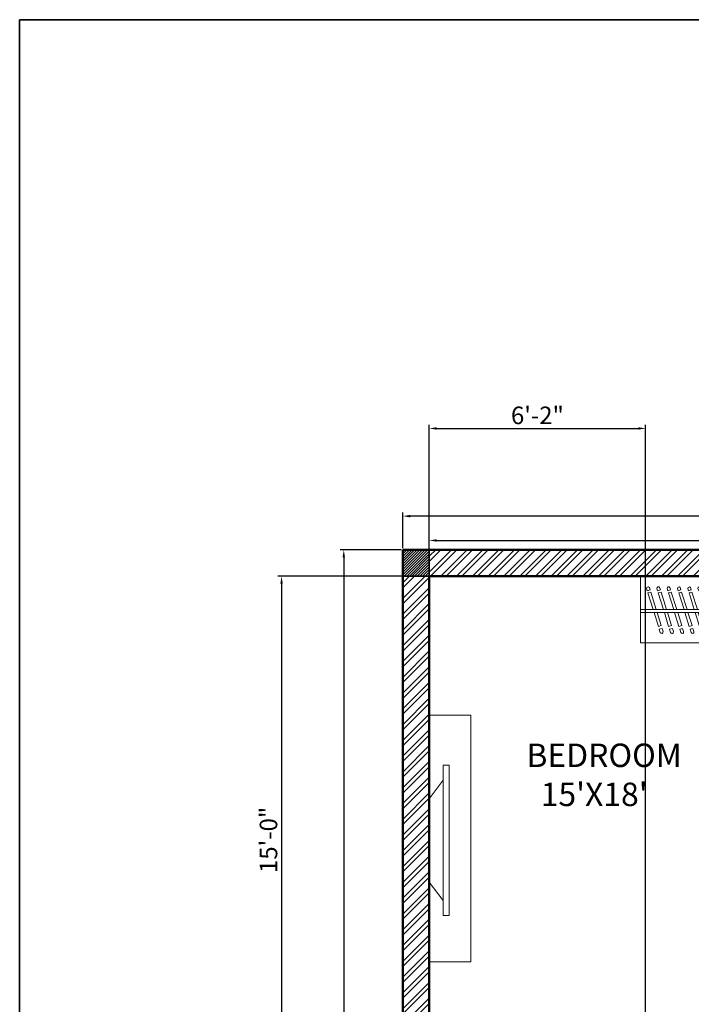
# Model space of a CAD drawing. Units: millimetres. Extents: x 20768 to 23556, y 50760 to 52704.
# Tile 21 of 36: x 20768 to 20998, y 52368 to 52704. Entities that reach past the tile are written whole.
import ezdxf

# ---------------------------------------------------------------- set-up
doc = ezdxf.new("R2010")
doc.units = ezdxf.units.MM
for name, color, linetype, lineweight in [('A-ANNO-DIMS', 2, 'Continuous', 18), ('A-ANNO-TTLB', 7, 'Continuous', 35), ('A-AREA-IDEN', 40, 'Continuous', 18), ('A-FURN', 8, 'Continuous', 18), ('A-WALL', 7, 'Continuous', 50), ('A-WALL-PATT', 8, 'Continuous', 13), ('S-ANNO-DIMS', 2, 'Continuous', 18), ('S-COLS', 20, 'Continuous', 35)]:
    doc.layers.add(name, color=color, linetype=linetype, lineweight=lineweight)
doc.styles.get("Standard").update_dxf_attribs({"font": 'arial.ttf'})
doc.dimstyles.new('ISO-25', dxfattribs={"dimtxt": 6, "dimasz": 2.5, "dimexe": 1.25, "dimexo": 0.625, "dimtad": 1, "dimdec": 0, "dimlunit": 3, "dimtxsty": 'Standard', "dimcen": 2.5, "dimadec": 0, "dimazin": 0, "dimtfac": 1, "dimtdec": 0, "dimtmove": 0, "dimatfit": 3, "dimfxl": 1, "dimarcsym": 0})
pattern_1 = [(45, (-81.1113, 0), (-2.69407684, 2.69407684), []), (45, (-79.3152, 0), (-2.69407684, 2.69407684), [])]

# ---------------------------------------------------------------- blocks, each defined once
blk = doc.blocks.new('wb')
for p, q in [((21205.25, 52502.52), (21061.44, 52502.52)), ((21205.25, 52501.52), (21061.44, 52501.52))]:
    blk.add_line(p, q)
blk.add_lwpolyline([(21205.25, 52513.9), (21061.44, 52513.9), (21061.44, 52491.15), (21205.25, 52491.15)], close=True)
for points in [[(21064.45, 52510.07, 0.695903), (21063.5, 52509.77), (21063.75, 52508.98), (21064.7, 52509.27)], [(21067.97, 52510.07, 0.695903), (21067.01, 52509.77), (21067.26, 52508.98), (21068.21, 52509.27)], [(21071.48, 52510.07, 0.695903), (21070.52, 52509.77), (21070.77, 52508.98), (21071.73, 52509.27)], [(21074.99, 52510.07, 0.695903), (21074.04, 52509.77), (21074.28, 52508.98), (21075.24, 52509.27)], [(21078.5, 52510.07, 0.695903), (21077.55, 52509.77), (21077.8, 52508.98), (21078.75, 52509.27)], [(21082.02, 52510.07, 0.695903), (21081.06, 52509.77), (21081.31, 52508.98), (21082.26, 52509.27)], [(21085.53, 52510.07, 0.695903), (21084.57, 52509.77), (21084.82, 52508.98), (21085.78, 52509.27)], [(21089.04, 52510.07, 0.695903), (21088.09, 52509.77), (21088.33, 52508.98), (21089.29, 52509.27)], [(21092.55, 52510.07, 0.695903), (21091.6, 52509.77), (21091.85, 52508.98), (21092.8, 52509.27)], [(21096.07, 52510.07, 0.695903), (21095.11, 52509.77), (21095.36, 52508.98), (21096.31, 52509.27)], [(21099.58, 52510.07, 0.695903), (21098.62, 52509.77), (21098.87, 52508.98), (21099.83, 52509.27)], [(21103.09, 52510.07, 0.695903), (21102.14, 52509.77), (21102.38, 52508.98), (21103.34, 52509.27)], [(21106.6, 52510.07, 0.695903), (21105.65, 52509.77), (21105.9, 52508.98), (21106.85, 52509.27)], [(21110.12, 52510.07, 0.695903), (21109.16, 52509.77), (21109.41, 52508.98), (21110.36, 52509.27)], [(21113.63, 52510.07, 0.695903), (21112.67, 52509.77), (21112.92, 52508.98), (21113.88, 52509.27)], [(21117.14, 52510.07, 0.695903), (21116.19, 52509.77), (21116.43, 52508.98), (21117.39, 52509.27)], [(21120.65, 52510.07, 0.695903), (21119.7, 52509.77), (21119.95, 52508.98), (21120.9, 52509.27)], [(21124.17, 52510.07, 0.695903), (21123.21, 52509.77), (21123.46, 52508.98), (21124.41, 52509.27)], [(21127.68, 52510.07, 0.695903), (21126.72, 52509.77), (21126.97, 52508.98), (21127.93, 52509.27)], [(21131.19, 52510.07, 0.695903), (21130.24, 52509.77), (21130.48, 52508.98), (21131.44, 52509.27)], [(21134.7, 52510.07, 0.695903), (21133.75, 52509.77), (21134, 52508.98), (21134.95, 52509.27)], [(21138.22, 52510.07, 0.695903), (21137.26, 52509.77), (21137.51, 52508.98), (21138.46, 52509.27)], [(21141.73, 52510.07, 0.695903), (21140.77, 52509.77), (21141.02, 52508.98), (21141.98, 52509.27)], [(21145.24, 52510.07, 0.695903), (21144.29, 52509.77), (21144.54, 52508.98), (21145.49, 52509.27)], [(21148.75, 52510.07, 0.695903), (21147.8, 52509.77), (21148.05, 52508.98), (21149, 52509.27)], [(21152.27, 52510.07, 0.695903), (21151.31, 52509.77), (21151.56, 52508.98), (21152.52, 52509.27)], [(21155.78, 52510.07, 0.695903), (21154.83, 52509.77), (21155.07, 52508.98), (21156.03, 52509.27)], [(21159.29, 52510.07, 0.695903), (21158.34, 52509.77), (21158.59, 52508.98), (21159.54, 52509.27)], [(21162.8, 52510.07, 0.695903), (21161.85, 52509.77), (21162.1, 52508.98), (21163.05, 52509.27)], [(21166.32, 52510.07, 0.695903), (21165.36, 52509.77), (21165.61, 52508.98), (21166.57, 52509.27)], [(21169.83, 52510.07, 0.695903), (21168.88, 52509.77), (21169.12, 52508.98), (21170.08, 52509.27)], [(21173.34, 52510.07, 0.695903), (21172.39, 52509.77), (21172.64, 52508.98), (21173.59, 52509.27)], [(21176.86, 52510.07, 0.695903), (21175.9, 52509.77), (21176.15, 52508.98), (21177.1, 52509.27)], [(21180.37, 52510.07, 0.695903), (21179.41, 52509.77), (21179.66, 52508.98), (21180.62, 52509.27)], [(21183.88, 52510.07, 0.695903), (21182.93, 52509.77), (21183.17, 52508.98), (21184.13, 52509.27)], [(21187.39, 52510.07, 0.695903), (21186.44, 52509.77), (21186.69, 52508.98), (21187.64, 52509.27)], [(21190.91, 52510.07, 0.695903), (21189.95, 52509.77), (21190.2, 52508.98), (21191.15, 52509.27)], [(21194.42, 52510.07, 0.695903), (21193.46, 52509.77), (21193.71, 52508.98), (21194.67, 52509.27)], [(21197.93, 52510.07, 0.695903), (21196.98, 52509.77), (21197.22, 52508.98), (21198.18, 52509.27)], [(21068.81, 52496.1), (21067.85, 52495.8), (21068.19, 52494.73, 1), (21069.14, 52495.03)], [(21072.32, 52496.1), (21071.37, 52495.8), (21071.7, 52494.73, 1), (21072.65, 52495.03)], [(21075.83, 52496.1), (21074.88, 52495.8), (21075.21, 52494.73, 1), (21076.17, 52495.03)], [(21079.35, 52496.1), (21078.39, 52495.8), (21078.73, 52494.73, 1), (21079.68, 52495.03)], [(21082.86, 52496.1), (21081.9, 52495.8), (21082.24, 52494.73, 1), (21083.19, 52495.03)], [(21086.37, 52496.1), (21085.42, 52495.8), (21085.75, 52494.73, 1), (21086.7, 52495.03)], [(21089.88, 52496.1), (21088.93, 52495.8), (21089.26, 52494.73, 1), (21090.22, 52495.03)], [(21093.4, 52496.1), (21092.44, 52495.8), (21092.78, 52494.73, 1), (21093.73, 52495.03)], [(21096.91, 52496.1), (21095.95, 52495.8), (21096.29, 52494.73, 1), (21097.24, 52495.03)], [(21100.42, 52496.1), (21099.47, 52495.8), (21099.8, 52494.73, 1), (21100.76, 52495.03)], [(21103.93, 52496.1), (21102.98, 52495.8), (21103.31, 52494.73, 1), (21104.27, 52495.03)], [(21107.45, 52496.1), (21106.49, 52495.8), (21106.83, 52494.73, 1), (21107.78, 52495.03)], [(21110.96, 52496.1), (21110, 52495.8), (21110.34, 52494.73, 1), (21111.29, 52495.03)], [(21114.47, 52496.1), (21113.52, 52495.8), (21113.85, 52494.73, 1), (21114.81, 52495.03)], [(21117.98, 52496.1), (21117.03, 52495.8), (21117.36, 52494.73, 1), (21118.32, 52495.03)], [(21121.5, 52496.1), (21120.54, 52495.8), (21120.88, 52494.73, 1), (21121.83, 52495.03)], [(21125.01, 52496.1), (21124.05, 52495.8), (21124.39, 52494.73, 1), (21125.34, 52495.03)], [(21128.52, 52496.1), (21127.57, 52495.8), (21127.9, 52494.73, 1), (21128.86, 52495.03)], [(21132.03, 52496.1), (21131.08, 52495.8), (21131.41, 52494.73, 1), (21132.37, 52495.03)], [(21135.55, 52496.1), (21134.59, 52495.8), (21134.93, 52494.73, 1), (21135.88, 52495.03)], [(21139.06, 52496.1), (21138.1, 52495.8), (21138.44, 52494.73, 1), (21139.39, 52495.03)], [(21142.57, 52496.1), (21141.62, 52495.8), (21141.95, 52494.73, 1), (21142.91, 52495.03)], [(21146.08, 52496.1), (21145.13, 52495.8), (21145.46, 52494.73, 1), (21146.42, 52495.03)], [(21149.6, 52496.1), (21148.64, 52495.8), (21148.98, 52494.73, 1), (21149.93, 52495.03)], [(21153.11, 52496.1), (21152.15, 52495.8), (21152.49, 52494.73, 1), (21153.44, 52495.03)], [(21156.62, 52496.1), (21155.67, 52495.8), (21156, 52494.73, 1), (21156.96, 52495.03)], [(21160.13, 52496.1), (21159.18, 52495.8), (21159.51, 52494.73, 1), (21160.47, 52495.03)], [(21163.65, 52496.1), (21162.69, 52495.8), (21163.03, 52494.73, 1), (21163.98, 52495.03)], [(21167.16, 52496.1), (21166.2, 52495.8), (21166.54, 52494.73, 1), (21167.49, 52495.03)], [(21170.67, 52496.1), (21169.72, 52495.8), (21170.05, 52494.73, 1), (21171.01, 52495.03)], [(21174.18, 52496.1), (21173.23, 52495.8), (21173.56, 52494.73, 1), (21174.52, 52495.03)], [(21177.7, 52496.1), (21176.74, 52495.8), (21177.08, 52494.73, 1), (21178.03, 52495.03)], [(21181.21, 52496.1), (21180.25, 52495.8), (21180.59, 52494.73, 1), (21181.54, 52495.03)], [(21184.72, 52496.1), (21183.77, 52495.8), (21184.1, 52494.73, 1), (21185.06, 52495.03)], [(21188.23, 52496.1), (21187.28, 52495.8), (21187.61, 52494.73, 1), (21188.57, 52495.03)], [(21191.75, 52496.1), (21190.79, 52495.8), (21191.13, 52494.73, 1), (21192.08, 52495.03)], [(21195.26, 52496.1), (21194.31, 52495.8), (21194.64, 52494.73, 1), (21195.59, 52495.03)], [(21198.77, 52496.1), (21197.82, 52495.8), (21198.15, 52494.73, 1), (21199.11, 52495.03)], [(21202.29, 52496.1), (21201.33, 52495.8), (21201.67, 52494.73, 1), (21202.62, 52495.03)]]:
    blk.add_lwpolyline(points, format="xyb", close=True)
for points in [[(21065.76, 52502.52), (21063.98, 52508.23), (21064.93, 52508.53), (21066.81, 52502.52)], [(21069.27, 52502.52), (21067.49, 52508.23), (21068.44, 52508.53), (21070.32, 52502.52)], [(21072.78, 52502.52), (21071, 52508.23), (21071.96, 52508.53), (21073.83, 52502.52)], [(21076.3, 52502.52), (21074.51, 52508.23), (21075.47, 52508.53), (21077.34, 52502.52)], [(21079.81, 52502.52), (21078.03, 52508.23), (21078.98, 52508.53), (21080.86, 52502.52)], [(21083.32, 52502.52), (21081.54, 52508.23), (21082.49, 52508.53), (21084.37, 52502.52)], [(21086.83, 52502.52), (21085.05, 52508.23), (21086.01, 52508.53), (21087.88, 52502.52)], [(21090.35, 52502.52), (21088.57, 52508.23), (21089.52, 52508.53), (21091.39, 52502.52)], [(21093.86, 52502.52), (21092.08, 52508.23), (21093.03, 52508.53), (21094.91, 52502.52)], [(21097.37, 52502.52), (21095.59, 52508.23), (21096.55, 52508.53), (21098.42, 52502.52)], [(21100.88, 52502.52), (21099.1, 52508.23), (21100.06, 52508.53), (21101.93, 52502.52)], [(21104.4, 52502.52), (21102.62, 52508.23), (21103.57, 52508.53), (21105.44, 52502.52)], [(21107.91, 52502.52), (21106.13, 52508.23), (21107.08, 52508.53), (21108.96, 52502.52)], [(21111.42, 52502.52), (21109.64, 52508.23), (21110.6, 52508.53), (21112.47, 52502.52)], [(21114.93, 52502.52), (21113.15, 52508.23), (21114.11, 52508.53), (21115.98, 52502.52)], [(21118.45, 52502.52), (21116.67, 52508.23), (21117.62, 52508.53), (21119.49, 52502.52)], [(21121.96, 52502.52), (21120.18, 52508.23), (21121.13, 52508.53), (21123.01, 52502.52)], [(21125.47, 52502.52), (21123.69, 52508.23), (21124.65, 52508.53), (21126.52, 52502.52)], [(21128.98, 52502.52), (21127.2, 52508.23), (21128.16, 52508.53), (21130.03, 52502.52)], [(21132.5, 52502.52), (21130.72, 52508.23), (21131.67, 52508.53), (21133.54, 52502.52)], [(21136.01, 52502.52), (21134.23, 52508.23), (21135.18, 52508.53), (21137.06, 52502.52)], [(21139.52, 52502.52), (21137.74, 52508.23), (21138.7, 52508.53), (21140.57, 52502.52)], [(21143.03, 52502.52), (21141.25, 52508.23), (21142.21, 52508.53), (21144.08, 52502.52)], [(21146.55, 52502.52), (21144.77, 52508.23), (21145.72, 52508.53), (21147.59, 52502.52)], [(21150.06, 52502.52), (21148.28, 52508.23), (21149.23, 52508.53), (21151.11, 52502.52)], [(21153.57, 52502.52), (21151.79, 52508.23), (21152.75, 52508.53), (21154.62, 52502.52)], [(21157.08, 52502.52), (21155.3, 52508.23), (21156.26, 52508.53), (21158.13, 52502.52)], [(21160.6, 52502.52), (21158.82, 52508.23), (21159.77, 52508.53), (21161.64, 52502.52)], [(21164.11, 52502.52), (21162.33, 52508.23), (21163.28, 52508.53), (21165.16, 52502.52)], [(21167.62, 52502.52), (21165.84, 52508.23), (21166.8, 52508.53), (21168.67, 52502.52)], [(21171.13, 52502.52), (21169.35, 52508.23), (21170.31, 52508.53), (21172.18, 52502.52)], [(21174.65, 52502.52), (21172.87, 52508.23), (21173.82, 52508.53), (21175.69, 52502.52)], [(21178.16, 52502.52), (21176.38, 52508.23), (21177.33, 52508.53), (21179.21, 52502.52)], [(21181.67, 52502.52), (21179.89, 52508.23), (21180.85, 52508.53), (21182.72, 52502.52)], [(21185.19, 52502.52), (21183.4, 52508.23), (21184.36, 52508.53), (21186.23, 52502.52)], [(21188.7, 52502.52), (21186.92, 52508.23), (21187.87, 52508.53), (21189.75, 52502.52)], [(21192.21, 52502.52), (21190.43, 52508.23), (21191.38, 52508.53), (21193.26, 52502.52)], [(21195.72, 52502.52), (21193.94, 52508.23), (21194.9, 52508.53), (21196.77, 52502.52)], [(21199.24, 52502.52), (21197.46, 52508.23), (21198.41, 52508.53), (21200.28, 52502.52)], [(21066.07, 52501.52), (21067.54, 52496.81), (21068.49, 52497.1), (21067.12, 52501.52)], [(21069.58, 52501.52), (21071.05, 52496.81), (21072.01, 52497.1), (21070.63, 52501.52)], [(21073.09, 52501.52), (21074.57, 52496.81), (21075.52, 52497.1), (21074.14, 52501.52)], [(21076.61, 52501.52), (21078.08, 52496.81), (21079.03, 52497.1), (21077.65, 52501.52)], [(21080.12, 52501.52), (21081.59, 52496.81), (21082.55, 52497.1), (21081.17, 52501.52)], [(21083.63, 52501.52), (21085.1, 52496.81), (21086.06, 52497.1), (21084.68, 52501.52)], [(21087.14, 52501.52), (21088.62, 52496.81), (21089.57, 52497.1), (21088.19, 52501.52)], [(21090.66, 52501.52), (21092.13, 52496.81), (21093.08, 52497.1), (21091.7, 52501.52)], [(21094.17, 52501.52), (21095.64, 52496.81), (21096.6, 52497.1), (21095.22, 52501.52)], [(21097.68, 52501.52), (21099.15, 52496.81), (21100.11, 52497.1), (21098.73, 52501.52)], [(21101.2, 52501.52), (21102.67, 52496.81), (21103.62, 52497.1), (21102.24, 52501.52)], [(21104.71, 52501.52), (21106.18, 52496.81), (21107.13, 52497.1), (21105.76, 52501.52)], [(21108.22, 52501.52), (21109.69, 52496.81), (21110.65, 52497.1), (21109.27, 52501.52)], [(21111.73, 52501.52), (21113.2, 52496.81), (21114.16, 52497.1), (21112.78, 52501.52)], [(21115.25, 52501.52), (21116.72, 52496.81), (21117.67, 52497.1), (21116.29, 52501.52)], [(21118.76, 52501.52), (21120.23, 52496.81), (21121.18, 52497.1), (21119.81, 52501.52)], [(21122.27, 52501.52), (21123.74, 52496.81), (21124.7, 52497.1), (21123.32, 52501.52)], [(21125.78, 52501.52), (21127.25, 52496.81), (21128.21, 52497.1), (21126.83, 52501.52)], [(21129.3, 52501.52), (21130.77, 52496.81), (21131.72, 52497.1), (21130.34, 52501.52)], [(21132.81, 52501.52), (21134.28, 52496.81), (21135.23, 52497.1), (21133.86, 52501.52)], [(21136.32, 52501.52), (21137.79, 52496.81), (21138.75, 52497.1), (21137.37, 52501.52)], [(21139.83, 52501.52), (21141.3, 52496.81), (21142.26, 52497.1), (21140.88, 52501.52)], [(21143.35, 52501.52), (21144.82, 52496.81), (21145.77, 52497.1), (21144.39, 52501.52)], [(21146.86, 52501.52), (21148.33, 52496.81), (21149.28, 52497.1), (21147.91, 52501.52)], [(21150.37, 52501.52), (21151.84, 52496.81), (21152.8, 52497.1), (21151.42, 52501.52)], [(21153.88, 52501.52), (21155.35, 52496.81), (21156.31, 52497.1), (21154.93, 52501.52)], [(21157.4, 52501.52), (21158.87, 52496.81), (21159.82, 52497.1), (21158.44, 52501.52)], [(21160.91, 52501.52), (21162.38, 52496.81), (21163.33, 52497.1), (21161.96, 52501.52)], [(21164.42, 52501.52), (21165.89, 52496.81), (21166.85, 52497.1), (21165.47, 52501.52)], [(21167.93, 52501.52), (21169.4, 52496.81), (21170.36, 52497.1), (21168.98, 52501.52)], [(21171.45, 52501.52), (21172.92, 52496.81), (21173.87, 52497.1), (21172.49, 52501.52)], [(21174.96, 52501.52), (21176.43, 52496.81), (21177.38, 52497.1), (21176.01, 52501.52)], [(21178.47, 52501.52), (21179.94, 52496.81), (21180.9, 52497.1), (21179.52, 52501.52)], [(21181.98, 52501.52), (21183.46, 52496.81), (21184.41, 52497.1), (21183.03, 52501.52)], [(21185.5, 52501.52), (21186.97, 52496.81), (21187.92, 52497.1), (21186.54, 52501.52)], [(21189.01, 52501.52), (21190.48, 52496.81), (21191.43, 52497.1), (21190.06, 52501.52)], [(21192.52, 52501.52), (21193.99, 52496.81), (21194.95, 52497.1), (21193.57, 52501.52)], [(21196.03, 52501.52), (21197.51, 52496.81), (21198.46, 52497.1), (21197.08, 52501.52)], [(21199.55, 52501.52), (21201.02, 52496.81), (21201.97, 52497.1), (21200.59, 52501.52)]]:
    blk.add_lwpolyline(points)
blk = doc.blocks.new('tv')
for p, q in [((20989.25, 52437.95), (20993.93, 52444.3)), ((20989.25, 52409.51), (20993.93, 52403.15))]:
    blk.add_line(p, q)
for points in [[(20989.25, 52466.51), (21003.46, 52466.51), (21003.46, 52382.21), (20989.25, 52382.21)], [(20993.93, 52449.42), (20996.05, 52449.42), (20996.05, 52398.03), (20993.93, 52398.03)]]:
    blk.add_lwpolyline(points, close=True)
blk = doc.blocks.new('*D108')
at = {"layer": 'A-ANNO-DIMS', "color": 0, "lineweight": -2, "transparency": 16777216}
for p, q in [((20898.51, 52522.9), (20877.66, 52522.9)), ((20878.91, 52520.4), (20878.91, 51832.4)), ((20898.51, 51829.9), (20877.66, 51829.9))]:
    blk.add_line(p, q, dxfattribs=at)
at = {"layer": 'A-ANNO-DIMS', "color": 0, "transparency": 16777216}
for points in [[(20878.49, 52520.4), (20879.33, 52520.4), (20878.91, 52522.9)], [(20878.49, 51832.4), (20879.33, 51832.4), (20878.91, 51829.9)]]:
    blk.add_solid(points, dxfattribs=at)
at = {"layer": 'Defpoints', "color": 0, "transparency": 16777216}
for p in [(20899.14, 52522.9), (20878.91, 51829.9), (20899.14, 51829.9)]:
    blk.add_point(p, dxfattribs=at)
at = {"layer": 'A-ANNO-DIMS', "color": 0, "transparency": 16777216, "insert": (20875.22, 52176.4), "char_height": 6, "attachment_point": 5, "rotation": 90}
blk.add_mtext('57\'-9"', dxfattribs=at)
blk = doc.blocks.new('*D109')
at = {"layer": 'A-ANNO-DIMS', "color": 0, "lineweight": -2, "transparency": 16777216}
for p, q in [((20899.14, 52523.52), (20899.14, 52535.7)), ((21130.64, 52534.45), (20901.64, 52534.45)), ((21133.14, 52523.52), (21133.14, 52535.7))]:
    blk.add_line(p, q, dxfattribs=at)
at = {"layer": 'A-ANNO-DIMS', "color": 0, "transparency": 16777216}
for points in [[(20901.64, 52534.87), (20901.64, 52534.03), (20899.14, 52534.45)], [(21130.64, 52534.87), (21130.64, 52534.03), (21133.14, 52534.45)]]:
    blk.add_solid(points, dxfattribs=at)
at = {"layer": 'Defpoints', "color": 0, "transparency": 16777216}
for p in [(20899.14, 52534.45), (20899.14, 52522.9), (21133.14, 52522.9)]:
    blk.add_point(p, dxfattribs=at)
at = {"layer": 'A-ANNO-DIMS', "color": 0, "transparency": 16777216, "insert": (21016.14, 52538.14), "char_height": 6, "attachment_point": 5}
blk.add_mtext('19\'-6"', dxfattribs=at)
blk = doc.blocks.new('*D110')
at = {"layer": 'A-ANNO-DIMS', "color": 0, "lineweight": -2, "transparency": 16777216}
for p, q in [((20908.14, 52523.52), (20908.14, 52527.41)), ((21124.14, 52523.52), (21124.14, 52527.41)), ((20910.64, 52526.16), (21121.64, 52526.16))]:
    blk.add_line(p, q, dxfattribs=at)
at = {"layer": 'A-ANNO-DIMS', "color": 0, "transparency": 16777216}
for points in [[(20910.64, 52526.57), (20910.64, 52525.74), (20908.14, 52526.16)], [(21121.64, 52526.57), (21121.64, 52525.74), (21124.14, 52526.16)]]:
    blk.add_solid(points, dxfattribs=at)
at = {"layer": 'Defpoints', "color": 0, "transparency": 16777216}
for p in [(21124.14, 52526.16), (20908.14, 52522.9), (21124.14, 52522.9)]:
    blk.add_point(p, dxfattribs=at)
at = {"layer": 'A-ANNO-DIMS', "color": 0, "transparency": 16777216, "insert": (21016.14, 52529.85), "char_height": 6, "attachment_point": 5}
blk.add_mtext("18'", dxfattribs=at)
blk = doc.blocks.new('*D201')
at = {"layer": 'Defpoints', "color": 0, "transparency": 16777216}
for p in [(20908.14, 52513.9), (20857.64, 52333.9), (20908.14, 52333.9)]:
    blk.add_point(p, dxfattribs=at)
at = {"layer": 'S-ANNO-DIMS', "color": 0, "lineweight": -2, "transparency": 16777216}
for p, q in [((20907.51, 52513.9), (20856.39, 52513.9)), ((20857.64, 52511.4), (20857.64, 52336.4)), ((20907.51, 52333.9), (20856.39, 52333.9))]:
    blk.add_line(p, q, dxfattribs=at)
at = {"layer": 'S-ANNO-DIMS', "color": 0, "transparency": 16777216}
for points in [[(20857.22, 52511.4), (20858.06, 52511.4), (20857.64, 52513.9)], [(20857.22, 52336.4), (20858.06, 52336.4), (20857.64, 52333.9)]]:
    blk.add_solid(points, dxfattribs=at)
at = {"layer": 'S-ANNO-DIMS', "color": 0, "transparency": 16777216, "insert": (20853.95, 52423.9), "char_height": 6, "attachment_point": 5, "rotation": 90}
blk.add_mtext('15\'-0"', dxfattribs=at)
blk = doc.blocks.new('*D209')
at = {"layer": 'Defpoints', "color": 0, "transparency": 16777216}
for p in [(20982.04, 52564.4), (20908.14, 52333.9), (20982.04, 52333.9)]:
    blk.add_point(p, dxfattribs=at)
at = {"layer": 'S-ANNO-DIMS', "color": 0, "lineweight": -2, "transparency": 16777216}
for p, q in [((20908.14, 52334.52), (20908.14, 52565.65)), ((20910.64, 52564.4), (20979.54, 52564.4)), ((20982.04, 52334.52), (20982.04, 52565.65))]:
    blk.add_line(p, q, dxfattribs=at)
at = {"layer": 'S-ANNO-DIMS', "color": 0, "transparency": 16777216}
for points in [[(20910.64, 52564.81), (20910.64, 52563.98), (20908.14, 52564.4)], [(20979.54, 52564.81), (20979.54, 52563.98), (20982.04, 52564.4)]]:
    blk.add_solid(points, dxfattribs=at)
at = {"layer": 'S-ANNO-DIMS', "color": 0, "transparency": 16777216, "insert": (20945.09, 52568.09), "char_height": 6, "attachment_point": 5}
blk.add_mtext('6\'-2"', dxfattribs=at)

msp = doc.modelspace()

# ---------------------------------------------------------------- hatches: boundary and pattern name
at = {"layer": 'A-WALL-PATT'}
h = msp.add_hatch(dxfattribs=at)
h.set_pattern_fill('ANSI31', color=256, scale=0.2)
h.set_pattern_definition([(45, (-81.11126, 0), (-0.449012806, 0.449012806), [])])
h.paths.add_polyline_path([(20908.14, 52522.9), (20899.14, 52522.9), (20899.14, 52513.9), (20908.14, 52513.9)])
h = msp.add_hatch(dxfattribs=at)
h.set_pattern_fill('ANSI32', color=256, scale=0.4)
h.set_pattern_definition(pattern_1)
h.paths.add_polyline_path([(21124.14, 52522.9), (20908.14, 52522.9), (20908.14, 52513.9), (21124.14, 52513.9)])
h = msp.add_hatch(dxfattribs=at)
h.set_pattern_fill('ANSI32', color=256, scale=0.4)
h.set_pattern_definition(pattern_1)
h.paths.add_polyline_path([(20908.14, 52513.9), (20899.14, 52513.9), (20899.14, 52335.9), (20908.14, 52335.9)])

# ---------------------------------------------------------------- linework, layer by layer
at = {"layer": 'A-ANNO-TTLB'}
msp.add_lwpolyline([(20768.14, 52703.98), (23555.8, 52703.98), (23555.8, 51623.53), (20768.14, 51623.53)], close=True, dxfattribs=at)
at = {"layer": 'A-WALL'}
for p, q in [((20899.14, 52522.9), (20899.14, 51829.9)), ((20899.14, 52522.9), (21133.14, 52522.9)), ((20908.14, 52513.9), (20908.14, 51838.9)), ((20908.14, 52513.9), (21124.14, 52513.9))]:
    msp.add_line(p, q, dxfattribs=at)
at = {"layer": 'S-COLS'}
msp.add_lwpolyline([(20908.14, 52513.9), (20899.14, 52513.9), (20899.14, 52522.9), (20908.14, 52522.9)], close=True, dxfattribs=at)

# ---------------------------------------------------------------- block references
at = {"layer": 'A-FURN'}
for name in ['wb', 'tv']:
    msp.add_blockref(name, (-81.11, 0), dxfattribs=at)

# ---------------------------------------------------------------- texts
at = {"layer": 'A-AREA-IDEN', "insert": (20941.32, 52456.78), "char_height": 8, "attachment_point": 1}
msp.add_mtext_dynamic_manual_height_columns("BEDROOM\\P  15'X18'", width=49.9521, gutter_width=12.5, heights=[0], dxfattribs=at)

# ---------------------------------------------------------------- dimensions: what is measured, and where the dimension line sits
at = {"layer": 'A-ANNO-DIMS'}
for base, p1, p2, picture, middle in [((20899.14, 52534.45), (21133.14, 52522.9), (20899.14, 52522.9), '*D109', (21016.14, 52538.14)), ((21124.14, 52526.16), (20908.14, 52522.9), (21124.14, 52522.9), '*D110', (21016.14, 52529.85))]:
    dim = msp.add_linear_dim(base=base, p1=p1, p2=p2, dimstyle='ISO-25', override={"dimclrd": 0, "dimclre": 0, "dimclrt": 0}, dxfattribs=at)
    dim.commit()
    dim.dimension.update_dxf_attribs({"geometry": picture, "text_midpoint": middle})
dim = msp.add_linear_dim(base=(20878.91, 51829.9), p1=(20899.14, 52522.9), p2=(20899.14, 51829.9), angle=90, dimstyle='ISO-25', override={"dimclrd": 0, "dimclre": 0, "dimclrt": 0}, dxfattribs=at)
dim.commit()
dim.dimension.update_dxf_attribs({"geometry": '*D108', "text_midpoint": (20875.22, 52176.4)})
at = {"layer": 'S-ANNO-DIMS'}
dim = msp.add_linear_dim(base=(20982.04, 52564.4), p1=(20908.14, 52333.9), p2=(20982.04, 52333.9), dimstyle='ISO-25', override={"dimdec": 1, "dimlfac": 1, "dimrnd": 0, "dimzin": 1, "dimdsep": 46, "dimlunit": 4, "dimfrac": 2}, dxfattribs=at)
dim.commit()
dim.dimension.update_dxf_attribs({"geometry": '*D209', "text_midpoint": (20945.09, 52568.09)})
dim = msp.add_linear_dim(base=(20857.64, 52333.9), p1=(20908.14, 52513.9), p2=(20908.14, 52333.9), angle=90, dimstyle='ISO-25', override={"dimdec": 1, "dimlfac": 1, "dimrnd": 0, "dimzin": 1, "dimdsep": 46, "dimlunit": 4, "dimfrac": 2}, dxfattribs=at)
dim.commit()
dim.dimension.update_dxf_attribs({"geometry": '*D201', "text_midpoint": (20853.95, 52423.9)})

doc.saveas('drawing.dxf')
